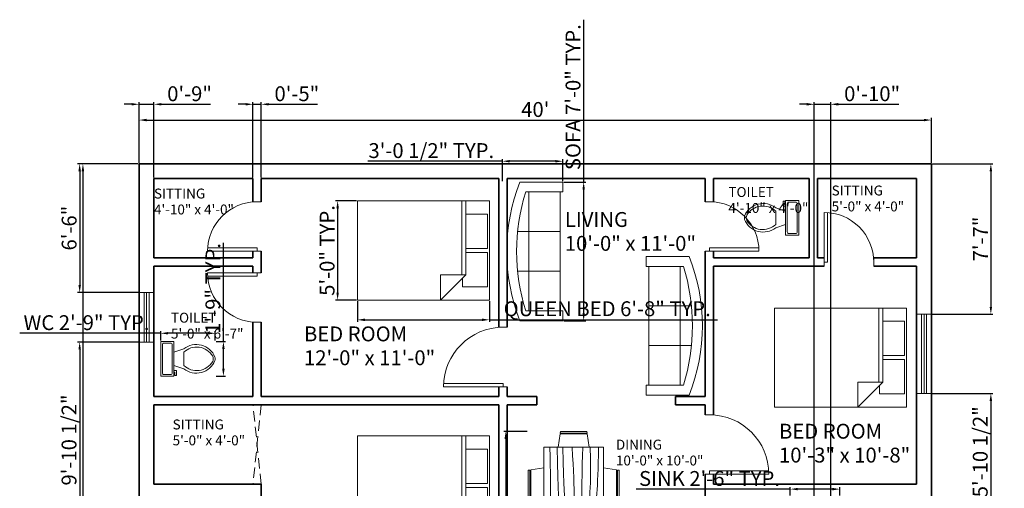
# Model space of a CAD drawing. Units: inches. Extents: x 3087 to 8148, y 1377 to 3709.
# Tile 6 of 6: x 3087 to 3684, y 1877 to 2161. Entities that reach past the tile are written whole.
import ezdxf

# ---------------------------------------------------------------- set-up
doc = ezdxf.new("R2010")
doc.units = ezdxf.units.IN
doc.linetypes.add('HIDDEN', pattern=[9.525, 6.35, -3.175])
for name, color, linetype, lineweight, true_color in [('A-ANNO-DIMS', 244, 'Continuous', 18, 0x991b1e), ('A-AREA-IDEN', 244, 'Continuous', 18, 0x991b1e), ('A-DOOR', 146, 'Continuous', 18, 0x105689), ('A-GLAZ', 146, 'Continuous', 18, 0x105689), ('A-WALL', 241, 'Continuous', 35, 0xf7abae), ('A-WALL-HIDN', 244, 'HIDDEN', 13, 0x991b1e)]:
    doc.layers.add(name, color=color, linetype=linetype, lineweight=lineweight, true_color=true_color)
doc.layers.add('A-FLOR-FIXT', color=9, linetype='Continuous', lineweight=18)
doc.layers.add('A-FURN', color=8, linetype='Continuous', lineweight=18)
doc.styles.get("Standard").update_dxf_attribs({"font": 'arial.ttf'})
doc.dimstyles.new('ISO-25', dxfattribs={"dimtxt": 9, "dimasz": 4.5, "dimexe": 1.25, "dimexo": 0.625, "dimtad": 1, "dimdec": 0, "dimlunit": 3, "dimtxsty": 'Standard', "dimcen": 2.5, "dimadec": 0, "dimazin": 0, "dimtfac": 1, "dimtdec": 0, "dimtmove": 0, "dimatfit": 3, "dimfxl": 1, "dimarcsym": 0})

# ---------------------------------------------------------------- blocks, each defined once
blk = doc.blocks.new('Bed - Queen')
for p, q in [((0, -80.00003), (0, 0)), ((0, 0), (59.99999, 0)), ((59.99999, 0), (59.99999, -80.00003)), ((7.99999, -1.2), (28.79998, -1.2)), ((7.99999, -14.4), (7.99999, -1.2)), ((28.79998, -1.2), (28.79998, -14.4)), ((31.19999, -1.2), (51.99999, -1.2)), ((31.19999, -14.4), (31.19999, -1.2)), ((51.99999, -1.2), (51.99999, -16.4)), ((0, -14.4), (44.8, -14.4)), ((44.8, -16.8), (0, -16.8)), ((59.99999, -29.6), (44.8, -14.4)), ((44.8, -14.4), (44.8, -29.6)), ((51.99999, -16.4), (46.79936, -16.4)), ((44.8, -29.6), (59.99999, -29.6)), ((59.99999, -80.00003), (0, -80.00003))]:
    blk.add_line(p, q)
blk = doc.blocks.new('Toilet - top')
for p, q in [((9.5, -6), (9.5, -2)), ((-10, -8.5), (-8, -8.5)), ((-10, -9.5), (-10, -8.5)), ((-7, -9.5), (-10, -9.5)), ((-8, -8.5), (-8, -8)), ((-7, -8), (-7, -9.5)), ((-4, -8), (-6, -14)), ((4, -8), (6, -14)), ((4, -14), (-4, -14))]:
    blk.add_line(p, q)
blk.add_lwpolyline([(10.5, -8), (10.5, 0), (-10.5, 0), (-10.5, -8)], close=True)
for points in [[(-9.5, -2), (-9.5, -6)], [(8.5, -1), (-8.5, -1)], [(-8.5, -7), (8.5, -7)]]:
    blk.add_lwpolyline(points)
for centre, radius, start, end in [((-8.62, -1.88), 0.884, 81.8699, 188.1301), ((8.62, -1.88), 0.884, 351.8699, 98.1301), ((-8.62, -6.12), 0.884, 171.8699, 278.1301), ((8.62, -6.12), 0.884, 261.8699, 8.1301), ((3.52, -21.58), 12.17, 141.46911, 247.97143), ((4.2, -21.82), 11.33, 136.36773, 238.94682), ((-3.52, -21.58), 12.17, 292.02843, 38.53071), ((-4.2, -21.82), 11.33, 301.05301, 43.63209), ((0, -27.88), 4, 245.73182, 294.26817), ((0, -29), 4, 254.86053, 285.13947)]:
    blk.add_arc(centre, radius, start, end)
blk = doc.blocks.new('Dining Set - 36 x 72 in.')
for p, q in [((-22.2343, 26.00059), (-23.4847, 17.99762)), ((-22.2304, 26), (-5.7608, 26)), ((-22, 27.5), (-22.1562, 26.50042)), ((-5.8416, 26.5), (-22.1534, 26.5)), ((-22, 27.5), (-6, 27.5)), ((-5.8437, 26.49966), (-6, 27.5)), ((-4.5152, 17.99762), (-5.7655, 25.99926)), ((5.7657, 26.00059), (4.5153, 17.99762)), ((5.7696, 26), (22.2392, 26)), ((6, 27.5), (5.8438, 26.50042)), ((22.1584, 26.5), (5.8466, 26.5)), ((6, 27.5), (22, 27.5)), ((22.1563, 26.49966), (22, 27.5)), ((23.4848, 17.99762), (22.2345, 25.99926)), ((36, 18), (-36, 18)), ((-36, 18), (-36, -18)), ((36, -18), (36, 18)), ((-45.5, 8), (-44.5004, 8.15617)), ((-45.5, 8), (-45.5, -8)), ((-44.5, -8.15843), (-44.5, 8.15338)), ((-44.0006, 8.23428), (-35.9976, 9.48474)), ((-44, 8.23041), (-44, -8.23915)), ((44.0006, 8.23428), (35.9976, 9.48474)), ((44, 8.23041), (44, -8.23915)), ((44.5, -8.15843), (44.5, 8.15338)), ((45.5, 8), (44.5005, 8.15617)), ((45.5, 8), (45.5, -8)), ((-44.4997, -8.15631), (-45.5, -8)), ((-35.9976, -9.48476), (-43.9993, -8.2345)), ((35.9976, -9.48476), (43.9993, -8.2345)), ((44.4997, -8.15631), (45.5, -8)), ((-36, -18), (36, -18)), ((-22.2343, -26.0006), (-23.4847, -17.99762)), ((-4.5152, -17.99762), (-5.7655, -25.99928)), ((5.7657, -26.0006), (4.5153, -17.99762)), ((23.4848, -17.99762), (22.2345, -25.99928)), ((-22.2304, -26), (-5.7608, -26)), ((-22, -27.5), (-22.1562, -26.50044)), ((-5.8416, -26.5), (-22.1534, -26.5)), ((-22, -27.5), (-6, -27.5)), ((-5.8437, -26.49967), (-6, -27.5)), ((5.7696, -26), (22.2392, -26)), ((6, -27.5), (5.8438, -26.50044)), ((22.1584, -26.5), (5.8466, -26.5)), ((6, -27.5), (22, -27.5)), ((22.1563, -26.49967), (22, -27.5))]:
    blk.add_line(p, q)
for points in [[(-36, 15), (-31.1772, 14.97754), (-26.8079, 14.91406), (-22.8538, 14.81543), (-19.276, 14.6875), (-16.0362, 14.53613), (-13.0957, 14.36718), (-10.4159, 14.18652), (-7.9583, 14), (-5.6904, 13.81315), (-3.6035, 13.63021), (-1.6954, 13.45508), (0.0365, 13.29166), (1.5945, 13.14388), (2.9811, 13.01562), (4.1988, 12.9108), (5.25, 12.83333), (6.1393, 12.78613), (6.8802, 12.76823), (7.4883, 12.77767), (7.9792, 12.8125), (8.3685, 12.87077), (8.6719, 12.95052), (8.9049, 13.0498), (9.0833, 13.16666), (9.2205, 13.29899), (9.3216, 13.44401), (9.3895, 13.59879), (9.4271, 13.76041), (9.4373, 13.92594), (9.4232, 14.09245), (9.3875, 14.257), (9.3333, 14.41666), (9.2638, 14.56917), (9.1836, 14.71484), (9.0975, 14.85465), (9.0104, 14.98958), (8.9272, 15.1206), (8.8529, 15.2487), (8.7922, 15.37483), (8.75, 15.5), (8.7305, 15.62467), (8.7344, 15.74739), (8.7617, 15.86621), (8.8125, 15.97916), (8.8867, 16.08431), (8.9844, 16.17968), (9.1055, 16.26334), (9.25, 16.33333), (9.4189, 16.38802), (9.6172, 16.42708), (9.8506, 16.45052), (10.125, 16.45833), (10.4463, 16.45052), (10.8203, 16.42708), (11.2529, 16.38802), (11.75, 16.33333), (12.3184, 16.26318), (12.9694, 16.17838), (13.7151, 16.07991), (14.5677, 15.96875), (15.5395, 15.84586), (16.6426, 15.71224), (17.8893, 15.56884), (19.2917, 15.41666), (20.859, 15.25667), (22.5879, 15.08984), (24.4721, 14.91715), (26.5052, 14.73958), (28.6809, 14.5581), (30.9929, 14.3737), (33.4347, 14.18733), (36, 14)], [(-36, 10), (-28.9766, 10.14274), (-23.1725, 10.20442), (-18.4241, 10.19775), (-14.5677, 10.13541), (-11.4399, 10.03011), (-8.877, 9.89453), (-6.7154, 9.74137), (-4.7917, 9.58333), (-2.9698, 9.43082), (-1.2246, 9.28515), (0.4415, 9.14534), (2.026, 9.01041), (3.5266, 8.87939), (4.9408, 8.7513), (6.266, 8.62516), (7.5, 8.5), (8.6411, 8.37549), (9.6914, 8.2539), (10.6538, 8.13818), (11.5312, 8.03125), (12.3267, 7.93603), (13.043, 7.85547), (13.6831, 7.79248), (14.25, 7.75), (14.7471, 7.7303), (15.1797, 7.73307), (15.5537, 7.75732), (15.875, 7.80208), (16.1494, 7.86637), (16.3828, 7.94922), (16.5811, 8.04964), (16.75, 8.16666), (16.8944, 8.29915), (17.0143, 8.44531), (17.1089, 8.60319), (17.1771, 8.77083), (17.218, 8.94629), (17.2305, 9.1276), (17.2137, 9.31282), (17.1667, 9.5), (17.0895, 9.6875), (16.987, 9.875), (16.8649, 10.0625), (16.7292, 10.25), (16.5856, 10.4375), (16.4401, 10.625), (16.2985, 10.8125), (16.1667, 11), (16.05, 11.18733), (15.9518, 11.3737), (15.8752, 11.5581), (15.8229, 11.73958), (15.798, 11.91715), (15.8034, 12.08984), (15.842, 12.25667), (15.9167, 12.41666), (16.0295, 12.56836), (16.1784, 12.70833), (16.3605, 12.83268), (16.5729, 12.9375), (16.8127, 13.01888), (17.0768, 13.07291), (17.3625, 13.0957), (17.6667, 13.08333), (17.9894, 13.03312), (18.3418, 12.94726), (18.7382, 12.82918), (19.1927, 12.68229), (19.7195, 12.51001), (20.3327, 12.31575), (21.0465, 12.10294), (21.875, 11.875), (22.8357, 11.63354), (23.959, 11.37304), (25.2786, 11.08618), (26.8282, 10.76562), (28.6414, 10.40405), (30.752, 9.99414), (33.1936, 9.52856), (36, 9)], [(-36, 5.5), (-30.7157, 5.3348), (-26.069, 5.20963), (-21.9946, 5.11767), (-18.4271, 5.05208), (-15.3009, 5.00602), (-12.5508, 4.97265), (-10.1112, 4.94515), (-7.9167, 4.91666), (-5.909, 4.88167), (-4.0586, 4.83984), (-2.3429, 4.79215), (-0.7396, 4.73958), (0.7739, 4.6831), (2.22, 4.6237), (3.6213, 4.56233), (5, 4.5), (6.373, 4.43782), (7.7344, 4.3776), (9.0723, 4.32129), (10.375, 4.27083), (11.6309, 4.22819), (12.8281, 4.19531), (13.9551, 4.17415), (15, 4.16666), (15.954, 4.17448), (16.819, 4.19791), (17.6001, 4.23698), (18.3021, 4.29166), (18.9299, 4.36198), (19.4883, 4.44791), (19.9823, 4.54948), (20.4167, 4.66666), (20.7969, 4.79899), (21.1302, 4.94401), (21.4245, 5.09879), (21.6875, 5.26041), (21.9271, 5.42594), (22.1511, 5.59245), (22.3672, 5.757), (22.5834, 5.91666), (22.8065, 6.06868), (23.0404, 6.21093), (23.2879, 6.34147), (23.5521, 6.45833), (23.8358, 6.55957), (24.142, 6.64323), (24.4735, 6.70735), (24.8334, 6.75), (25.2235, 6.76969), (25.642, 6.76692), (26.0858, 6.74267), (26.5521, 6.69791), (27.0379, 6.63362), (27.5404, 6.55078), (28.0565, 6.45036), (28.5834, 6.33333), (29.1242, 6.19987), (29.7071, 6.04687), (30.3661, 5.87044), (31.1354, 5.66666), (32.0493, 5.43164), (33.142, 5.16146), (34.4475, 4.85221), (36, 4.5)], [(-36, -1), (-30.7915, -0.6591), (-26.0195, -0.38216), (-21.6519, -0.16284), (-17.6563, 0.00521), (-14.0005, 0.12833), (-10.6523, 0.21289), (-7.5796, 0.26522), (-4.75, 0.29166), (-2.134, 0.29793), (0.2878, 0.28711), (2.5317, 0.26163), (4.6146, 0.22396), (6.5529, 0.17651), (8.3633, 0.12174), (10.0623, 0.06209), (11.6667, 0), (13.1899, -0.06201), (14.6341, -0.1211), (15.9982, -0.17432), (17.2813, -0.21875), (18.4823, -0.25147), (19.6003, -0.26953), (20.6343, -0.27002), (21.5834, -0.25), (22.4481, -0.20768), (23.2357, -0.14584), (23.9549, -0.06836), (24.6146, 0.02083), (25.2235, 0.11784), (25.7904, 0.21875), (26.3241, 0.31966), (26.8334, 0.41666), (27.3265, 0.50618), (27.8099, 0.58593), (28.2894, 0.65397), (28.7709, 0.70833), (29.2601, 0.74707), (29.763, 0.76823), (30.2855, 0.76985), (30.8334, 0.75), (31.4088, 0.70784), (31.9994, 0.64713), (32.589, 0.57275), (33.1615, 0.48958), (33.7008, 0.4025), (34.1908, 0.3164), (34.6153, 0.23616), (34.9584, 0.16666), (35.2099, 0.11165), (35.3848, 0.07031), (35.504, 0.04069), (35.5886, 0.02083), (35.6594, 0.00879), (35.7377, 0.0026), (35.8442, 0.00032), (36, 0)], [(-36, -6.5), (-27.1843, -6.31267), (-20.084, -6.1263), (-14.469, -5.9419), (-10.1094, -5.76042), (-6.7752, -5.58285), (-4.2363, -5.41016), (-2.2629, -5.24333), (-0.625, -5.08334), (0.8708, -4.93099), (2.2715, -4.78646), (3.5872, -4.64974), (4.8281, -4.52084), (6.0046, -4.39974), (7.127, -4.28646), (8.2053, -4.18099), (9.25, -4.08334), (10.2705, -3.99382), (11.2734, -3.91407), (12.2647, -3.84603), (13.25, -3.79167), (14.2354, -3.75293), (15.2266, -3.73177), (16.2295, -3.73015), (17.25, -3.75), (18.2912, -3.79248), (19.3451, -3.85547), (20.4009, -3.93604), (21.4479, -4.03125), (22.4754, -4.13819), (23.4727, -4.25391), (24.4289, -4.37549), (25.3334, -4.5), (26.1785, -4.62492), (26.9694, -4.74935), (27.7145, -4.87281), (28.4219, -4.99479), (29.1, -5.11483), (29.7572, -5.23242), (30.4016, -5.34709), (31.0417, -5.45834), (31.6837, -5.56437), (32.3262, -5.65821), (32.9658, -5.73153), (33.599, -5.77604), (34.2224, -5.78345), (34.8327, -5.74545), (35.4264, -5.65373), (36, -5.5)], [(-36, -10), (-26.4022, -9.81299), (-18.4675, -9.62891), (-11.9839, -9.45069), (-6.7396, -9.28125), (-2.5226, -9.12354), (0.8789, -8.98047), (3.6769, -8.85498), (6.0833, -8.75), (8.2767, -8.66765), (10.3021, -8.60677), (12.1712, -8.56543), (13.8958, -8.54167), (15.4876, -8.53353), (16.9583, -8.53907), (18.3197, -8.55632), (19.5834, -8.58334), (20.7616, -8.61841), (21.8685, -8.66081), (22.9188, -8.71004), (23.9271, -8.76563), (24.9081, -8.82707), (25.8763, -8.89388), (26.8465, -8.96558), (27.8334, -9.04167), (28.8474, -9.12118), (29.8828, -9.20117), (30.93, -9.27824), (31.9792, -9.34896), (33.0205, -9.40991), (34.0443, -9.45768), (35.0407, -9.48885), (36, -9.5)], [(-36, -14.5), (-30.0881, -14.33513), (-25.0332, -14.21224), (-20.7312, -14.12647), (-17.0781, -14.07292), (-13.97, -14.04671), (-11.3027, -14.04297), (-8.9724, -14.05681), (-6.875, -14.08334), (-4.9224, -14.11833), (-3.0905, -14.16016), (-1.3709, -14.20785), (0.2448, -14.26042), (1.7647, -14.3169), (3.1973, -14.3763), (4.5507, -14.43767), (5.8333, -14.5), (7.0554, -14.5621), (8.235, -14.62175), (9.3922, -14.67652), (10.5469, -14.72396), (11.7192, -14.76164), (12.929, -14.78711), (14.1965, -14.79794), (15.5417, -14.79167), (16.9933, -14.76424), (18.6152, -14.70508), (20.4804, -14.60197), (22.6615, -14.44271), (25.2312, -14.21509), (28.2624, -13.9069), (31.8277, -13.50594), (36, -13)]]:
    blk.add_lwpolyline(points)
blk = doc.blocks.new('Sofa - Roundback 7 ft.')
for p, q in [((-36.000027, -34), (-36.000027, -11.4696)), ((-12.00002, -32.4421), (-12.00003, -6.5971)), ((11.99997, -32.4421), (11.99998, -6.5971)), ((35.99998, -34), (35.99998, -11.4696)), ((-35.999844, -13.3819), (35.9998, -13.3819)), ((-36.000027, -32.4421), (35.99998, -32.4421))]:
    blk.add_line(p, q)
for points in [[(-36.000027, -34), (-42.000027, -34), (-42.000027, -8)], [(41.99998, -8), (41.99998, -34), (35.99998, -34)]]:
    blk.add_lwpolyline(points)
for centre, radius, start, end in [((0, -114.25), 114.25, 68.43141, 111.5686), ((-0.00001, -127.1968), 121.1968, 72.72033, 107.2797)]:
    blk.add_arc(centre, radius, start, end)
blk = doc.blocks.new('*D17')
at = {"layer": 'A-ANNO-DIMS', "color": 0, "lineweight": -2, "transparency": 16777216}
for p, q in [((3159.82, 2074.59), (3159.82, 2101.66)), ((3164.32, 2100.41), (3635.32, 2100.41)), ((3639.82, 2074.59), (3639.82, 2101.66))]:
    blk.add_line(p, q, dxfattribs=at)
at = {"layer": 'A-ANNO-DIMS', "color": 0, "transparency": 16777216}
for points in [[(3164.32, 2101.16), (3164.32, 2099.66), (3159.82, 2100.41)], [(3635.32, 2101.16), (3635.32, 2099.66), (3639.82, 2100.41)]]:
    blk.add_solid(points, dxfattribs=at)
at = {"layer": 'Defpoints', "color": 0, "transparency": 16777216}
for p in [(3639.82, 2100.41), (3159.82, 2073.96), (3639.82, 2073.96)]:
    blk.add_point(p, dxfattribs=at)
at = {"layer": 'A-ANNO-DIMS', "color": 0, "transparency": 16777216, "insert": (3399.82, 2105.63), "char_height": 9, "attachment_point": 5}
blk.add_mtext("40'", dxfattribs=at)
blk = doc.blocks.new('*D18')
at = {"layer": 'A-ANNO-DIMS', "color": 0, "lineweight": -2, "transparency": 16777216}
for p, q in [((3159.19, 2073.96), (3124.53, 2073.96)), ((3125.78, 2069.46), (3125.78, 1418.46)), ((3159.19, 1413.96), (3124.53, 1413.96))]:
    blk.add_line(p, q, dxfattribs=at)
at = {"layer": 'A-ANNO-DIMS', "color": 0, "transparency": 16777216}
for points in [[(3125.03, 2069.46), (3126.53, 2069.46), (3125.78, 2073.96)], [(3125.03, 1418.46), (3126.53, 1418.46), (3125.78, 1413.96)]]:
    blk.add_solid(points, dxfattribs=at)
at = {"layer": 'Defpoints', "color": 0, "transparency": 16777216}
for p in [(3159.82, 2073.96), (3125.78, 1413.96), (3159.82, 1413.96)]:
    blk.add_point(p, dxfattribs=at)
at = {"layer": 'A-ANNO-DIMS', "color": 0, "transparency": 16777216, "insert": (3120.58, 1743.96), "char_height": 9, "attachment_point": 5, "rotation": 90}
blk.add_mtext("55'", dxfattribs=at)
blk = doc.blocks.new('DOOR-SINGLE-30IN')
for p, q in [((0, 30), (30, 30)), ((30, 30), (30, 28)), ((0, 28), (30, 28))]:
    blk.add_line(p, q)
blk.add_arc((30, 30), 30, 180, 270)
blk = doc.blocks.new('DOOR-SINGLE-36IN')
for p, q in [((0, 2), (36, 2)), ((36, 0), (36, 2)), ((0, 0), (36, 0))]:
    blk.add_line(p, q)
blk.add_arc((36, 0), 36, 90, 180)
blk = doc.blocks.new('WINDOW-30IN')
for p, q in [((0, 0), (0, 30)), ((9, 30), (0, 30)), ((3, 30), (3, 0)), ((4.5, 30), (4.5, 0)), ((6, 30), (6, 0)), ((9, 30), (9, 0)), ((9, 0), (0, 0))]:
    blk.add_line(p, q)
blk = doc.blocks.new('WINDOW-48IN')
for p, q in [((0, 0), (0, 48)), ((0, 48), (9, 48)), ((3, 0), (3, 48)), ((4.5, 0), (4.5, 48)), ((6, 0), (6, 48)), ((9, 48), (9, 0)), ((9, 0), (0, 0))]:
    blk.add_line(p, q)
blk = doc.blocks.new('*D31')
at = {"layer": 'A-ANNO-DIMS', "color": 0, "lineweight": -2, "transparency": 16777216}
for p, q in [((3292.09, 1990.84), (3292.09, 1978.21)), ((3372.09, 1990.84), (3372.09, 1978.21)), ((3296.59, 1979.46), (3367.59, 1979.46)), ((3372.09, 1979.46), (3510.23, 1979.46))]:
    blk.add_line(p, q, dxfattribs=at)
at = {"layer": 'A-ANNO-DIMS', "color": 0, "transparency": 16777216}
for points in [[(3296.59, 1980.21), (3296.59, 1978.71), (3292.09, 1979.46)], [(3367.59, 1980.21), (3367.59, 1978.71), (3372.09, 1979.46)]]:
    blk.add_solid(points, dxfattribs=at)
at = {"layer": 'Defpoints', "color": 0, "transparency": 16777216}
for p in [(3292.09, 1991.46), (3372.09, 1991.46), (3372.09, 1979.46)]:
    blk.add_point(p, dxfattribs=at)
at = {"layer": 'A-ANNO-DIMS', "color": 0, "transparency": 16777216, "insert": (3443.41, 1985.01), "char_height": 9, "attachment_point": 5}
blk.add_mtext('QUEEN BED 6\'-8" TYP.', dxfattribs=at)
blk = doc.blocks.new('*D32')
at = {"layer": 'A-ANNO-DIMS', "color": 0, "lineweight": -2, "transparency": 16777216}
for p, q in [((3291.47, 2051.46), (3278.84, 2051.46)), ((3280.09, 2046.96), (3280.09, 1995.96)), ((3291.47, 1991.46), (3278.84, 1991.46))]:
    blk.add_line(p, q, dxfattribs=at)
at = {"layer": 'A-ANNO-DIMS', "color": 0, "transparency": 16777216}
for points in [[(3279.34, 2046.96), (3280.84, 2046.96), (3280.09, 2051.46)], [(3279.34, 1995.96), (3280.84, 1995.96), (3280.09, 1991.46)]]:
    blk.add_solid(points, dxfattribs=at)
at = {"layer": 'Defpoints', "color": 0, "transparency": 16777216}
for p in [(3292.09, 2051.46), (3280.09, 1991.46), (3292.09, 1991.46)]:
    blk.add_point(p, dxfattribs=at)
at = {"layer": 'A-ANNO-DIMS', "color": 0, "transparency": 16777216, "insert": (3274.87, 2021.46), "char_height": 9, "attachment_point": 5, "rotation": 90}
blk.add_mtext('5\'-0" TYP.', dxfattribs=at)
blk = doc.blocks.new('*D33')
at = {"layer": 'A-ANNO-DIMS', "color": 0, "lineweight": -2, "transparency": 16777216}
for p, q in [((3172.9, 1971.31), (3087.49, 1971.31)), ((3172.9, 1966.97), (3172.9, 1972.56)), ((3201.45, 1971.31), (3177.4, 1971.31)), ((3205.95, 1966.97), (3205.95, 1972.56))]:
    blk.add_line(p, q, dxfattribs=at)
at = {"layer": 'A-ANNO-DIMS', "color": 0, "transparency": 16777216}
for points in [[(3177.4, 1972.06), (3177.4, 1970.56), (3172.9, 1971.31)], [(3201.45, 1972.06), (3201.45, 1970.56), (3205.95, 1971.31)]]:
    blk.add_solid(points, dxfattribs=at)
at = {"layer": 'Defpoints', "color": 0, "transparency": 16777216}
for p in [(3172.9, 1971.31), (3172.9, 1966.35), (3205.95, 1966.35)]:
    blk.add_point(p, dxfattribs=at)
at = {"layer": 'A-ANNO-DIMS', "color": 0, "transparency": 16777216, "insert": (3127.95, 1976.58), "char_height": 9, "attachment_point": 5}
blk.add_mtext('WC 2\'-9" TYP.', dxfattribs=at)
blk = doc.blocks.new('*D34')
at = {"layer": 'A-ANNO-DIMS', "color": 0, "lineweight": -2, "transparency": 16777216}
for p, q in [((3210.91, 1966.35), (3210.91, 2026.11)), ((3206.58, 1966.35), (3212.16, 1966.35)), ((3210.91, 1949.85), (3210.91, 1961.85)), ((3206.58, 1945.35), (3212.16, 1945.35))]:
    blk.add_line(p, q, dxfattribs=at)
at = {"layer": 'A-ANNO-DIMS', "color": 0, "transparency": 16777216}
for points in [[(3210.16, 1961.85), (3211.66, 1961.85), (3210.91, 1966.35)], [(3210.16, 1949.85), (3211.66, 1949.85), (3210.91, 1945.35)]]:
    blk.add_solid(points, dxfattribs=at)
at = {"layer": 'Defpoints', "color": 0, "transparency": 16777216}
for p in [(3205.95, 1966.35), (3210.91, 1966.35), (3205.95, 1945.35)]:
    blk.add_point(p, dxfattribs=at)
at = {"layer": 'A-ANNO-DIMS', "color": 0, "transparency": 16777216, "insert": (3205.69, 1998.48), "char_height": 9, "attachment_point": 5, "rotation": 90}
blk.add_mtext('1\'-9" TYP.', dxfattribs=at)
blk = doc.blocks.new('*D35')
at = {"layer": 'A-ANNO-DIMS', "color": 0, "lineweight": -2, "transparency": 16777216}
for p, q in [((3429.14, 2062.87), (3429.14, 2161.16)), ((3417.16, 2062.87), (3430.39, 2062.87)), ((3429.14, 1983.37), (3429.14, 2058.37)), ((3417.16, 1978.87), (3430.39, 1978.87))]:
    blk.add_line(p, q, dxfattribs=at)
at = {"layer": 'A-ANNO-DIMS', "color": 0, "transparency": 16777216}
for points in [[(3428.39, 2058.37), (3429.89, 2058.37), (3429.14, 2062.87)], [(3428.39, 1983.37), (3429.89, 1983.37), (3429.14, 1978.87)]]:
    blk.add_solid(points, dxfattribs=at)
at = {"layer": 'Defpoints', "color": 0, "transparency": 16777216}
for p in [(3416.54, 2062.87), (3429.14, 2062.87), (3416.54, 1978.87)]:
    blk.add_point(p, dxfattribs=at)
at = {"layer": 'A-ANNO-DIMS', "color": 0, "transparency": 16777216, "insert": (3423.86, 2114.27), "char_height": 9, "attachment_point": 5, "rotation": 90}
blk.add_mtext('SOFA 7\'-0" TYP.', dxfattribs=at)
blk = doc.blocks.new('*D36')
at = {"layer": 'A-ANNO-DIMS', "color": 0, "lineweight": -2, "transparency": 16777216}
for p, q in [((3379.87, 2063.5), (3379.87, 2076.72)), ((3416.54, 2063.5), (3416.54, 2076.72)), ((3379.87, 2075.47), (3298.3, 2075.47)), ((3412.04, 2075.47), (3384.37, 2075.47))]:
    blk.add_line(p, q, dxfattribs=at)
at = {"layer": 'A-ANNO-DIMS', "color": 0, "transparency": 16777216}
for points in [[(3384.37, 2076.22), (3384.37, 2074.72), (3379.87, 2075.47)], [(3412.04, 2076.22), (3412.04, 2074.72), (3416.54, 2075.47)]]:
    blk.add_solid(points, dxfattribs=at)
at = {"layer": 'Defpoints', "color": 0, "transparency": 16777216}
for p in [(3379.87, 2075.47), (3379.87, 2062.87), (3416.54, 2062.87)]:
    blk.add_point(p, dxfattribs=at)
at = {"layer": 'A-ANNO-DIMS', "color": 0, "transparency": 16777216, "insert": (3336.83, 2080.75), "char_height": 9, "attachment_point": 5}
blk.add_mtext('3\'-0 1/2" TYP.', dxfattribs=at)
blk = doc.blocks.new('*D41')
at = {"layer": 'A-ANNO-DIMS', "color": 0, "lineweight": -2, "transparency": 16777216}
for p, q in [((3394.96, 1911.86), (3380.68, 1911.86)), ((3381.93, 1907.36), (3381.93, 1825.36)), ((3394.96, 1820.86), (3380.68, 1820.86)), ((3381.93, 1820.86), (3381.93, 1685.25))]:
    blk.add_line(p, q, dxfattribs=at)
at = {"layer": 'A-ANNO-DIMS', "color": 0, "transparency": 16777216}
for points in [[(3381.18, 1907.36), (3382.68, 1907.36), (3381.93, 1911.86)], [(3381.18, 1825.36), (3382.68, 1825.36), (3381.93, 1820.86)]]:
    blk.add_solid(points, dxfattribs=at)
at = {"layer": 'Defpoints', "color": 0, "transparency": 16777216}
for p in [(3395.58, 1911.86), (3381.93, 1820.86), (3395.58, 1820.86)]:
    blk.add_point(p, dxfattribs=at)
at = {"layer": 'A-ANNO-DIMS', "color": 0, "transparency": 16777216, "insert": (3376.65, 1750.81), "char_height": 9, "attachment_point": 5, "rotation": 90}
blk.add_mtext('DINING SET 7\'-7" TYP.', dxfattribs=at)
blk = doc.blocks.new('*D47')
at = {"layer": 'A-ANNO-DIMS', "color": 0, "lineweight": -2, "transparency": 16777216}
for p, q in [((3554.32, 1876.96), (3460.91, 1876.96)), ((3554.32, 1873.09), (3554.32, 1878.21)), ((3579.82, 1876.96), (3558.82, 1876.96)), ((3584.32, 1873.09), (3584.32, 1878.21))]:
    blk.add_line(p, q, dxfattribs=at)
at = {"layer": 'A-ANNO-DIMS', "color": 0, "transparency": 16777216}
for points in [[(3558.82, 1877.71), (3558.82, 1876.21), (3554.32, 1876.96)], [(3579.82, 1877.71), (3579.82, 1876.21), (3584.32, 1876.96)]]:
    blk.add_solid(points, dxfattribs=at)
at = {"layer": 'Defpoints', "color": 0, "transparency": 16777216}
for p in [(3554.32, 1876.96), (3554.32, 1872.46), (3584.32, 1872.46)]:
    blk.add_point(p, dxfattribs=at)
at = {"layer": 'A-ANNO-DIMS', "color": 0, "transparency": 16777216, "insert": (3505.37, 1882.24), "char_height": 9, "attachment_point": 5}
blk.add_mtext('SINK 2\'-6" TYP.', dxfattribs=at)
blk = doc.blocks.new('*D59')
at = {"layer": 'A-ANNO-DIMS', "color": 0, "lineweight": -2, "transparency": 16777216}
for p, q in [((3155.32, 2109.96), (3150.82, 2109.96)), ((3159.82, 2074.59), (3159.82, 2111.21)), ((3159.82, 2109.96), (3168.82, 2109.96)), ((3168.82, 2065.59), (3168.82, 2111.21)), ((3173.32, 2109.96), (3202.99, 2109.96))]:
    blk.add_line(p, q, dxfattribs=at)
at = {"layer": 'A-ANNO-DIMS', "color": 0, "transparency": 16777216}
for points in [[(3155.32, 2110.71), (3155.32, 2109.21), (3159.82, 2109.96)], [(3173.32, 2110.71), (3173.32, 2109.21), (3168.82, 2109.96)]]:
    blk.add_solid(points, dxfattribs=at)
at = {"layer": 'Defpoints', "color": 0, "transparency": 16777216}
for p in [(3168.82, 2109.96), (3159.82, 2073.96), (3168.82, 2064.96)]:
    blk.add_point(p, dxfattribs=at)
at = {"layer": 'A-ANNO-DIMS', "color": 0, "transparency": 16777216, "insert": (3190.4, 2115.18), "char_height": 9, "attachment_point": 5}
blk.add_mtext('0\'-9"', dxfattribs=at)
blk = doc.blocks.new('*D60')
at = {"layer": 'A-ANNO-DIMS', "color": 0, "lineweight": -2, "transparency": 16777216}
for p, q in [((3224.32, 2109.96), (3219.82, 2109.96)), ((3228.82, 2065.59), (3228.82, 2111.21)), ((3228.82, 2109.96), (3233.82, 2109.96)), ((3233.82, 2065.59), (3233.82, 2111.21)), ((3238.32, 2109.96), (3267.99, 2109.96))]:
    blk.add_line(p, q, dxfattribs=at)
at = {"layer": 'A-ANNO-DIMS', "color": 0, "transparency": 16777216}
for points in [[(3224.32, 2110.71), (3224.32, 2109.21), (3228.82, 2109.96)], [(3238.32, 2110.71), (3238.32, 2109.21), (3233.82, 2109.96)]]:
    blk.add_solid(points, dxfattribs=at)
at = {"layer": 'Defpoints', "color": 0, "transparency": 16777216}
for p in [(3233.82, 2109.96), (3228.82, 2064.96), (3233.82, 2064.96)]:
    blk.add_point(p, dxfattribs=at)
at = {"layer": 'A-ANNO-DIMS', "color": 0, "transparency": 16777216, "insert": (3255.4, 2115.18), "char_height": 9, "attachment_point": 5}
blk.add_mtext('0\'-5"', dxfattribs=at)
blk = doc.blocks.new('*D61')
at = {"layer": 'A-ANNO-DIMS', "color": 0, "lineweight": -2, "transparency": 16777216}
for p, q in [((3159.19, 2073.96), (3122.57, 2073.96)), ((3123.82, 2069.46), (3123.82, 2000.51)), ((3159.19, 1996.01), (3122.57, 1996.01))]:
    blk.add_line(p, q, dxfattribs=at)
at = {"layer": 'A-ANNO-DIMS', "color": 0, "transparency": 16777216}
for points in [[(3123.07, 2069.46), (3124.57, 2069.46), (3123.82, 2073.96)], [(3123.07, 2000.51), (3124.57, 2000.51), (3123.82, 1996.01)]]:
    blk.add_solid(points, dxfattribs=at)
at = {"layer": 'Defpoints', "color": 0, "transparency": 16777216}
for p in [(3159.82, 2073.96), (3123.82, 1996.01), (3159.82, 1996.01)]:
    blk.add_point(p, dxfattribs=at)
at = {"layer": 'A-ANNO-DIMS', "color": 0, "transparency": 16777216, "insert": (3118.6, 2034.99), "char_height": 9, "attachment_point": 5, "rotation": 90}
blk.add_mtext('6\'-6"', dxfattribs=at)
blk = doc.blocks.new('*D62')
at = {"layer": 'A-ANNO-DIMS', "color": 0, "lineweight": -2, "transparency": 16777216}
for p, q in [((3159.19, 1966.01), (3122.57, 1966.01)), ((3123.82, 1961.51), (3123.82, 1851.89)), ((3159.19, 1847.39), (3122.57, 1847.39))]:
    blk.add_line(p, q, dxfattribs=at)
at = {"layer": 'A-ANNO-DIMS', "color": 0, "transparency": 16777216}
for points in [[(3123.07, 1961.51), (3124.57, 1961.51), (3123.82, 1966.01)], [(3123.07, 1851.89), (3124.57, 1851.89), (3123.82, 1847.39)]]:
    blk.add_solid(points, dxfattribs=at)
at = {"layer": 'Defpoints', "color": 0, "transparency": 16777216}
for p in [(3159.82, 1966.01), (3123.82, 1847.39), (3159.82, 1847.39)]:
    blk.add_point(p, dxfattribs=at)
at = {"layer": 'A-ANNO-DIMS', "color": 0, "transparency": 16777216, "insert": (3118.54, 1906.7), "char_height": 9, "attachment_point": 5, "rotation": 90}
blk.add_mtext('9\'-10 1/2"', dxfattribs=at)
blk = doc.blocks.new('*D65')
at = {"layer": 'A-ANNO-DIMS', "color": 0, "lineweight": -2, "transparency": 16777216}
for p, q in [((3640.442588, 2073.960564), (3677.067588, 2073.960564)), ((3675.817588, 2069.460564), (3675.817588, 1987.317068)), ((3640.442588, 1982.817068), (3677.067588, 1982.817068))]:
    blk.add_line(p, q, dxfattribs=at)
at = {"layer": 'A-ANNO-DIMS', "color": 0, "transparency": 16777216}
for points in [[(3675.067588, 2069.460564), (3676.567588, 2069.460564), (3675.817588, 2073.960564)], [(3675.067588, 1987.317068), (3676.567588, 1987.317068), (3675.817588, 1982.817068)]]:
    blk.add_solid(points, dxfattribs=at)
at = {"layer": 'Defpoints', "color": 0, "transparency": 16777216}
for p in [(3639.817588, 2073.960564), (3639.817588, 1982.817068), (3675.817588, 1982.817068)]:
    blk.add_point(p, dxfattribs=at)
at = {"layer": 'A-ANNO-DIMS', "color": 0, "transparency": 16777216, "insert": (3670.692588, 2028.388816), "char_height": 9, "attachment_point": 5, "rotation": 90}
blk.add_mtext('7\'-7"', dxfattribs=at)
blk = doc.blocks.new('*D66')
at = {"layer": 'A-ANNO-DIMS', "color": 0, "lineweight": -2, "transparency": 16777216}
for p, q in [((3640.44, 1934.82), (3677.07, 1934.82)), ((3675.82, 1930.32), (3675.82, 1868.83)), ((3640.44, 1864.33), (3677.07, 1864.33))]:
    blk.add_line(p, q, dxfattribs=at)
at = {"layer": 'A-ANNO-DIMS', "color": 0, "transparency": 16777216}
for points in [[(3675.07, 1930.32), (3676.57, 1930.32), (3675.82, 1934.82)], [(3675.07, 1868.83), (3676.57, 1868.83), (3675.82, 1864.33)]]:
    blk.add_solid(points, dxfattribs=at)
at = {"layer": 'Defpoints', "color": 0, "transparency": 16777216}
for p in [(3639.82, 1934.82), (3639.82, 1864.33), (3675.82, 1864.33)]:
    blk.add_point(p, dxfattribs=at)
at = {"layer": 'A-ANNO-DIMS', "color": 0, "transparency": 16777216, "insert": (3670.54, 1899.58), "char_height": 9, "attachment_point": 5, "rotation": 90}
blk.add_mtext('5\'-10 1/2"', dxfattribs=at)
blk = doc.blocks.new('*D70')
at = {"layer": 'A-ANNO-DIMS', "color": 0, "lineweight": -2, "transparency": 16777216}
for p, q in [((3564.32, 2109.96), (3559.82, 2109.96)), ((3568.82, 1749.59), (3568.82, 2111.21)), ((3568.82, 2109.96), (3578.82, 2109.96)), ((3578.82, 1749.59), (3578.82, 2111.21)), ((3583.32, 2109.96), (3619.98, 2109.96))]:
    blk.add_line(p, q, dxfattribs=at)
at = {"layer": 'A-ANNO-DIMS', "color": 0, "transparency": 16777216}
for points in [[(3564.32, 2110.71), (3564.32, 2109.21), (3568.82, 2109.96)], [(3583.32, 2110.71), (3583.32, 2109.21), (3578.82, 2109.96)]]:
    blk.add_solid(points, dxfattribs=at)
at = {"layer": 'Defpoints', "color": 0, "transparency": 16777216}
for p in [(3578.82, 2109.96), (3568.82, 1748.96), (3578.82, 1748.96)]:
    blk.add_point(p, dxfattribs=at)
at = {"layer": 'A-ANNO-DIMS', "color": 0, "transparency": 16777216, "insert": (3603.9, 2115.18), "char_height": 9, "attachment_point": 5}
blk.add_mtext('0\'-10"', dxfattribs=at)

msp = doc.modelspace()

# ---------------------------------------------------------------- linework, layer by layer
at = {"layer": 'A-DOOR'}
for p, q in [((3228.82, 2050.96), (3233.82, 2050.96)), ((3502.82, 2050.96), (3507.82, 2050.96)), ((3228.82, 2020.96), (3233.82, 2020.96)), ((3502.82, 2020.96), (3507.82, 2020.96)), ((3574.82, 2016.96), (3574.82, 2011.96)), ((3604.82, 2016.96), (3604.82, 2011.96)), ((3228.82, 2007.96), (3233.82, 2007.96)), ((3228.82, 1977.96), (3233.82, 1977.96)), ((3377.82, 1974.96), (3382.82, 1974.96)), ((3377.82, 1938.96), (3382.82, 1938.96)), ((3502.82, 1921.96), (3507.82, 1921.96)), ((3502.82, 1885.96), (3507.82, 1885.96))]:
    msp.add_line(p, q, dxfattribs=at)
at = {"layer": 'A-WALL'}
for p, q in [((3159.82, 2073.96), (3639.82, 2073.96)), ((3159.82, 1413.96), (3159.82, 2073.96)), ((3639.82, 2073.96), (3639.82, 1413.96)), ((3168.82, 2064.96), (3228.82, 2064.96)), ((3168.82, 2016.96), (3168.82, 2064.96)), ((3228.82, 2050.96), (3228.82, 2064.96)), ((3233.82, 2050.96), (3233.82, 2064.96)), ((3233.82, 2064.96), (3377.82, 2064.96)), ((3377.82, 1974.96), (3377.82, 2064.96)), ((3382.82, 1974.96), (3382.82, 2064.96)), ((3382.82, 2064.96), (3502.82, 2064.96)), ((3502.82, 2050.96), (3502.82, 2064.96)), ((3507.82, 2050.96), (3507.82, 2064.96)), ((3507.82, 2064.96), (3565.82, 2064.96)), ((3565.82, 2064.96), (3565.82, 2016.96)), ((3570.82, 2064.96), (3570.82, 2016.96)), ((3570.82, 2064.96), (3630.82, 2064.96)), ((3630.82, 2064.96), (3630.82, 2016.96)), ((3168.82, 2016.96), (3228.82, 2016.96)), ((3228.82, 2016.96), (3228.82, 2020.96)), ((3233.82, 2007.96), (3233.82, 2020.96)), ((3502.82, 1932.96), (3502.82, 2020.96)), ((3507.82, 2016.96), (3507.82, 2020.96)), ((3507.82, 2016.96), (3565.82, 2016.96)), ((3570.82, 2016.96), (3574.82, 2016.96)), ((3604.82, 2016.96), (3630.82, 2016.96)), ((3168.82, 2011.96), (3228.82, 2011.96)), ((3168.82, 1932.96), (3168.82, 2011.96)), ((3228.82, 2007.96), (3228.82, 2011.96)), ((3507.82, 2011.96), (3574.82, 2011.96)), ((3507.82, 1921.96), (3507.82, 2011.96)), ((3604.82, 2011.96), (3630.82, 2011.96)), ((3630.82, 2011.96), (3630.82, 1879.96)), ((3228.82, 1932.96), (3228.82, 1977.96)), ((3233.82, 1932.96), (3233.82, 1977.96)), ((3377.82, 1932.96), (3377.82, 1938.96)), ((3382.82, 1932.96), (3382.82, 1938.96)), ((3168.82, 1932.96), (3228.82, 1932.96)), ((3233.82, 1932.96), (3377.82, 1932.96)), ((3382.82, 1932.96), (3400.82, 1932.96)), ((3400.82, 1927.96), (3400.82, 1932.96)), ((3484.82, 1927.96), (3484.82, 1932.96)), ((3484.82, 1932.96), (3502.82, 1932.96)), ((3168.82, 1927.96), (3233.82, 1927.96)), ((3168.82, 1879.96), (3168.82, 1927.96)), ((3233.82, 1927.96), (3377.82, 1927.96)), ((3377.82, 1807.96), (3377.82, 1927.96)), ((3382.82, 1807.96), (3382.82, 1927.96)), ((3382.82, 1927.96), (3400.82, 1927.96)), ((3484.82, 1927.96), (3502.82, 1927.96)), ((3502.82, 1921.96), (3502.82, 1927.96)), ((3502.82, 1870.96), (3502.82, 1885.96)), ((3507.82, 1879.96), (3507.82, 1885.96)), ((3168.82, 1879.96), (3233.82, 1879.96)), ((3233.82, 1807.96), (3233.82, 1879.96)), ((3507.82, 1879.96), (3630.82, 1879.96))]:
    msp.add_line(p, q, dxfattribs=at)
at = {"layer": 'A-WALL-HIDN'}
for p, q in [((3233.82, 1927.96), (3228.82, 1879.96)), ((3233.82, 1879.96), (3228.82, 1927.96))]:
    msp.add_line(p, q, dxfattribs=at)

# ---------------------------------------------------------------- block references
at = {"layer": 'A-DOOR', "extrusion": (0, 0, -1), "zscale": -1}
for p, rotation in [((-3201.32, 2050.96), 180), ((-3604.82, 2044.46), 269.9999999999994)]:
    msp.add_blockref('DOOR-SINGLE-30IN', p, dxfattribs=dict(at, rotation=rotation))
at = {"layer": 'A-DOOR', "rotation": 180}
msp.add_blockref('DOOR-SINGLE-30IN', (3535.32, 2050.96), dxfattribs=at)
at = {"layer": 'A-DOOR'}
for name, p in [('DOOR-SINGLE-30IN', (3201.32, 1977.96)), ('DOOR-SINGLE-36IN', (3344.32, 1938.96))]:
    msp.add_blockref(name, p, dxfattribs=at)
at = {"layer": 'A-DOOR', "extrusion": (0, 0, -1), "zscale": -1}
msp.add_blockref('DOOR-SINGLE-36IN', (-3541.32, 1885.96), dxfattribs=at)
at = {"layer": 'A-FLOR-FIXT'}
for p, rotation in [((3559.49, 2041.23), 270), ((3172.9, 1955.85), 90)]:
    msp.add_blockref('Toilet - top', p, dxfattribs=dict(at, rotation=rotation))
at = {"layer": 'A-FURN'}
for name, p, rotation in [('Sofa - Roundback 7 ft.', (3382.54, 2020.87), 89.99999999999999), ('Bed - Queen', (3372.09, 2051.46), 270), ('Sofa - Roundback 7 ft.', (3501.03, 1975.84), 270), ('Bed - Queen', (3624.75, 1986.56), 270), ('Bed - Queen', (3372.09, 1909.14), 270), ('Dining Set - 36 x 72 in.', (3423.08, 1866.36), 269.9999999999999)]:
    msp.add_blockref(name, p, dxfattribs=dict(at, rotation=rotation))
at = {"layer": 'A-GLAZ'}
for name, p in [('WINDOW-30IN', (3159.82, 1966.01)), ('WINDOW-48IN', (3630.82, 1934.82))]:
    msp.add_blockref(name, p, dxfattribs=at)

# ---------------------------------------------------------------- texts
at = {"layer": 'A-AREA-IDEN'}
for s, height, p in [('SITTING', 6, (3168.82, 2052.91)), ('TOILET ', 6, (3516.83, 2053.83)), ('SITTING', 6, (3579.36, 2054.75)), ('4\'-10" x 4\'-0"', 6, (3168.82, 2043.27)), ('4\'-10" x 4\'-0"', 6, (3516.83, 2044.19)), ('5\'-0" x 4\'-0"', 6, (3579.36, 2045.11)), ('LIVING', 9, (3417.72, 2035.7)), ('10\'-0" x 11\'-0"', 9, (3417.72, 2021.24)), ('TOILET ', 6, (3179.14, 1977.75)), ('5\'-0" x 6\'-7"', 6, (3179.14, 1968.11)), ('BED ROOM ', 9, (3259.73, 1966.45)), ('12\'-0" x 11\'-0"', 9, (3259.73, 1951.99)), ('SITTING', 6, (3180.12, 1913.1)), ('BED ROOM ', 9, (3547.49, 1907.51)), ('5\'-0" x 4\'-0"', 6, (3180.12, 1903.46)), ('DINING ', 6, (3448.68, 1900.91)), ('10\'-0" x 10\'-0"', 6, (3448.68, 1891.27)), ('10\'-3" x 10\'-8"', 9, (3547.49, 1893.06))]:
    msp.add_text(s, height=height, dxfattribs=at).set_placement(p)

# ---------------------------------------------------------------- dimensions: what is measured, and where the dimension line sits
at = {"layer": 'A-ANNO-DIMS'}
for base, p1, p2, angle, text, picture, middle in [((3429.14, 2062.87), (3416.54, 1978.87), (3416.54, 2062.87), 90, 'SOFA <> TYP.', '*D35', (3423.86, 2114.27)), ((3379.87, 2075.47), (3416.54, 2062.87), (3379.87, 2062.87), 180, '<> TYP.', '*D36', (3336.83, 2080.75)), ((3280.09, 1991.46), (3292.09, 2051.46), (3292.09, 1991.46), 270, '<> TYP.', '*D32', (3274.87, 2021.46)), ((3210.91, 1966.35), (3205.95, 1945.35), (3205.95, 1966.35), 90, '<> TYP.', '*D34', (3205.69, 1998.48)), ((3172.904, 1971.3054), (3205.9502, 1966.3484), (3172.904, 1966.3484), 180, 'WC <> TYP.', '*D33', (3127.9451, 1976.5838)), ((3381.93, 1820.86), (3395.58, 1911.86), (3395.58, 1820.86), 270, 'DINING SET <> TYP.', '*D41', (3376.65, 1750.81)), ((3554.32, 1876.96), (3584.32, 1872.46), (3554.32, 1872.46), 180, 'SINK <> TYP.', '*D47', (3505.37, 1882.24))]:
    dim = msp.add_linear_dim(base=base, p1=p1, p2=p2, angle=angle, text=text, dimstyle='ISO-25', override={"dimdec": 1, "dimlfac": 1, "dimrnd": 0, "dimzin": 1, "dimdsep": 46, "dimlunit": 4, "dimfrac": 2}, dxfattribs=at)
    dim.commit()
    dim.dimension.update_dxf_attribs({"geometry": picture, "text_midpoint": middle})
for base, p1, p2, override, picture, middle in [((3168.82, 2109.96), (3159.82, 2073.96), (3168.82, 2064.96), {"dimdec": 1, "dimlfac": 1, "dimrnd": 0, "dimzin": 1, "dimdsep": 46, "dimlunit": 4, "dimfrac": 2}, '*D59', (3190.4, 2115.18)), ((3233.82, 2109.96), (3228.82, 2064.96), (3233.82, 2064.96), {"dimdec": 1, "dimlfac": 1, "dimrnd": 0, "dimzin": 1, "dimdsep": 46, "dimlunit": 4, "dimfrac": 2}, '*D60', (3255.4, 2115.18)), ((3578.82, 2109.96), (3568.82, 1748.96), (3578.82, 1748.96), {"dimdec": 1, "dimlfac": 1, "dimrnd": 0, "dimzin": 1, "dimdsep": 46, "dimlunit": 4, "dimfrac": 2}, '*D70', (3603.9, 2115.18)), ((3639.82, 2100.41), (3159.82, 2073.96), (3639.82, 2073.96), {"dimclrd": 0, "dimclre": 0, "dimclrt": 0}, '*D17', (3399.82, 2105.63))]:
    dim = msp.add_linear_dim(base=base, p1=p1, p2=p2, dimstyle='ISO-25', override=override, dxfattribs=at)
    dim.commit()
    dim.dimension.update_dxf_attribs({"geometry": picture, "text_midpoint": middle})
for base, p1, p2, override, picture, middle in [((3123.8176, 1996.0104), (3159.8176, 2073.9606), (3159.8176, 1996.0104), {"dimdec": 1, "dimlfac": 1, "dimrnd": 0, "dimzin": 1, "dimdsep": 46, "dimlunit": 4, "dimfrac": 2}, '*D61', (3118.5974, 2034.9855)), ((3125.78, 1413.96), (3159.82, 2073.96), (3159.82, 1413.96), {"dimclrd": 0, "dimclre": 0, "dimclrt": 0}, '*D18', (3120.58, 1743.96)), ((3675.82, 1982.82), (3639.82, 2073.96), (3639.82, 1982.82), {"dimdec": 1, "dimlfac": 1, "dimrnd": 0, "dimzin": 1, "dimdsep": 46, "dimlunit": 4, "dimfrac": 2}, '*D65', (3670.69, 2028.39)), ((3123.82, 1847.39), (3159.82, 1966.01), (3159.82, 1847.39), {"dimdec": 1, "dimlfac": 1, "dimrnd": 0, "dimzin": 1, "dimdsep": 46, "dimlunit": 4, "dimfrac": 2}, '*D62', (3118.54, 1906.7)), ((3675.82, 1864.33), (3639.82, 1934.82), (3639.82, 1864.33), {"dimdec": 1, "dimlfac": 1, "dimrnd": 0, "dimzin": 1, "dimdsep": 46, "dimlunit": 4, "dimfrac": 2}, '*D66', (3670.54, 1899.58))]:
    dim = msp.add_linear_dim(base=base, p1=p1, p2=p2, angle=90, dimstyle='ISO-25', override=override, dxfattribs=at)
    dim.commit()
    dim.dimension.update_dxf_attribs({"geometry": picture, "text_midpoint": middle})
dim = msp.add_linear_dim(base=(3372.09, 1979.46), p1=(3292.09, 1991.46), p2=(3372.09, 1991.46), text='QUEEN BED <> TYP.', dimstyle='ISO-25', override={"dimdec": 1, "dimlfac": 1, "dimrnd": 0, "dimzin": 1, "dimdsep": 46, "dimlunit": 4, "dimfrac": 2}, dxfattribs=at)
dim.commit()
dim.dimension.update_dxf_attribs({"geometry": '*D31', "text_midpoint": (3443.41, 1985.01)})

doc.saveas('drawing.dxf')
